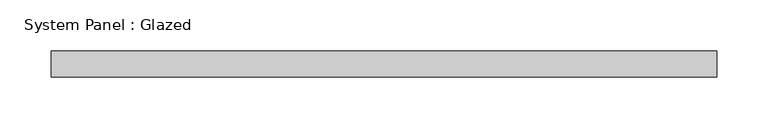
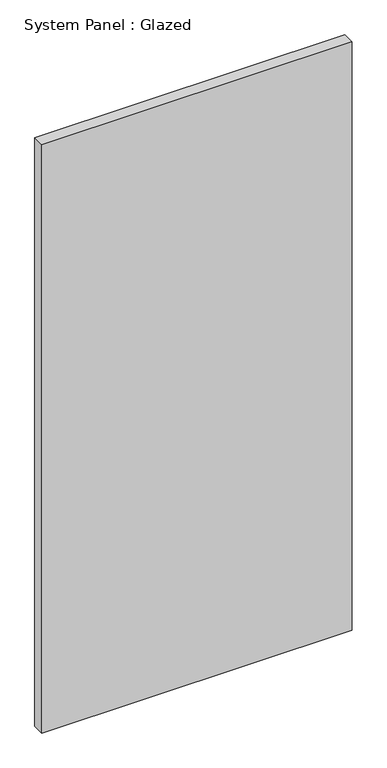
"""IFC4 building model written with IfcOpenShell, lengths in millimetres: plate geometry, System Panel : Glazed."""

from ifc_helpers import new_model, si_unit, origin, origin_with_axes, place, context, project, spatial, polyline, outline, extrude, source, transform, mapped, element, save


def system_panel_glazed_fafcfa65(model_context):
    return source(origin(), model_context, "Body", "SweptSolid", [
        extrude(outline(polyline([(323.85, 19.05), (-323.85, 19.05), (-323.85, 44.45), (323.85, 44.45), (323.85, 19.05)])), origin_with_axes(), (0.0, 0.0, 1.0), 1298.0105727),
    ])


if __name__ == "__main__":
    model = new_model("IFC4")
    model_context = context("Model", 3, world=origin())
    ifc_project = project(units=[si_unit("LENGTHUNIT", "METRE", prefix="MILLI")], contexts=[model_context])
    site = spatial("IfcSite", under=ifc_project)
    building = spatial("IfcBuilding", under=site)
    placement = place(None, origin())
    system_panel_glazed_shape = system_panel_glazed_fafcfa65(model_context)
    element("IfcPlate", 1, ObjectType="System Panel : Glazed", at=placement, inside=building, context=model_context, shape_type="MappedRepresentation", body=[
        mapped(system_panel_glazed_shape, transform((0.0, 0.0, 0.0), x_axis=(1.0, 0.0, 0.0), y_axis=(0.0, 1.0, 0.0), z_axis=(0.0, 0.0, 1.0))),
    ])
    save(model, "model.ifc")

# Revit data of these elements
# Type "System Panel : Glazed"
#   Construction Type Id = "GSP4R"
#   Analytic Construction = "1/8 in Pilkington single glazing"
#   Visual Light Transmittance = 0.9
#   Solar Heat Gain Coefficient = 0.86
#   Heat Transfer Coefficient (U) = 1.18115 BTU/(h·ft²·°F)
#   Define Thermal Properties by = 1
# Element 1 (IfcPlate, "System Panel : Glazed")
#   Materials on its faces: "Glass"
# Materials
#   "Glass": class "Glass", colour RGB 0 128 192, transparency 0.75, Description = "Soda Lime Glass", Cost = 0
